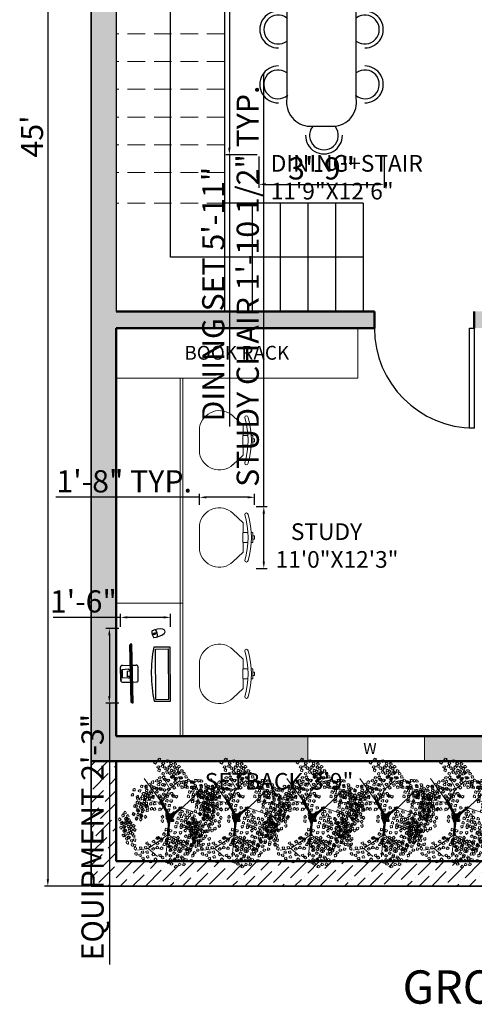
# Model space of a CAD drawing. Units: inches. Extents: x 3354 to 4308, y 1668 to 2317.
# Tile 1 of 11: x 3370 to 3534, y 1712 to 2066. Entities that reach past the tile are written whole.
import ezdxf

# ---------------------------------------------------------------- set-up
doc = ezdxf.new("R2010")
doc.units = ezdxf.units.IN
doc.linetypes.add('DASHED', pattern=[19.05, 12.7, -6.35])
for name, color, linetype, lineweight in [('A-ANNO-DIMS', 2, 'Continuous', 18), ('A-ANNO-TEXT', 7, 'Continuous', 18), ('A-AREA-IDEN', 3, 'Continuous', 18), ('A-DOOR', 3, 'Continuous', 25), ('A-EQPM', 9, 'Continuous', 18), ('A-FLOR-OVHD', 8, 'DASHED', 18), ('A-FLOR-STRS', 7, 'Continuous', 25), ('A-FURN', 8, 'Continuous', 18), ('A-GLAZ', 4, 'Continuous', 18), ('A-WALL', 7, 'Continuous', 50), ('A-WALL-PATT', 8, 'Continuous', 13), ('C-PROP', 1, 'Continuous', 35), ('L-PLNT', 84, 'Continuous', 13)]:
    doc.layers.add(name, color=color, linetype=linetype, lineweight=lineweight)
doc.layers.add('furniture', color=7, linetype='Continuous')
doc.layers.add('window', color=130, linetype='Continuous')
doc.styles.get("Standard").update_dxf_attribs({"font": 'arial.ttf'})
doc.dimstyles.new('ISO-25', dxfattribs={"dimtxt": 8, "dimasz": 2.5, "dimexe": 1.25, "dimexo": 0.625, "dimtad": 1, "dimdec": 1, "dimlunit": 3, "dimtxsty": 'Standard', "dimcen": 2.5, "dimadec": 0, "dimazin": 0, "dimtfac": 1, "dimtdec": 1, "dimtmove": 0, "dimatfit": 3, "dimfxl": 1, "dimarcsym": 0})

# ---------------------------------------------------------------- blocks, each defined once
blk = doc.blocks.new('*U3')
for p, q in [((0, 0), (0, -6)), ((36, 0), (36, -6))]:
    blk.add_line(p, q)
blk.add_lwpolyline([(0, 0), (0, 36), (1.75, 36), (1.75, 0)], close=True)
blk.add_arc((0, 0), 36, 0, 90)
blk = doc.blocks.new('UHYG')
at = {"color": 0}
for p, q in [((3464.1176, 1823.4027), (3464.1234, 1823.3981)), ((3464.1302, 1822.865), (3464.1358, 1822.8699))]:
    blk.add_line(p, q, dxfattribs=at)
at = {"layer": 'window'}
for p, q in [((3463.7616, 1823.3847), (3463.7651, 1822.8921)), ((3463.8967, 1823.3694), (3463.7767, 1823.3685)), ((3463.7767, 1823.3685), (3463.78, 1822.9085)), ((3463.8967, 1823.3694), (3463.9, 1822.9094)), ((3464.1234, 1823.3981), (3464.1358, 1822.8699)), ((3464.1078, 1823.2108), (3464.0735, 1823.21)), ((3464.1993, 1823.2129), (3464.1278, 1823.2112)), ((3464.1577, 1823.1587), (3464.1291, 1823.158)), ((3464.1576, 1823.1593), (3464.1356, 1823.1588)), ((3464.147, 1823.1745), (3464.2031, 1823.1717)), ((3464.1548, 1823.1586), (3464.1559, 1823.1106)), ((3464.1576, 1823.1593), (3464.1577, 1823.1587)), ((3464.2033, 1823.1649), (3464.2004, 1823.1649)), ((3464.2033, 1823.1643), (3464.201, 1823.1643)), ((3464.1114, 1823.0563), (3464.0771, 1823.0555)), ((3464.1588, 1823.1106), (3464.1302, 1823.11)), ((3464.2029, 1823.0584), (3464.1314, 1823.0568)), ((3464.1588, 1823.1101), (3464.1368, 1823.1096)), ((3464.1488, 1823.0943), (3464.2048, 1823.0998)), ((3464.1588, 1823.1106), (3464.1588, 1823.1101)), ((3464.2047, 1823.1066), (3464.2018, 1823.1065)), ((3464.2047, 1823.1071), (3464.2024, 1823.1071)), ((3463.9, 1822.9094), (3463.78, 1822.9085)), ((3463.8855, 1822.7631), (3463.8976, 1822.7664)), ((3463.9169, 1822.7716), (3463.8976, 1822.7664)), ((3463.9004, 1822.7713), (3463.912, 1822.7744)), ((3463.9025, 1822.7636), (3463.9141, 1822.7667)), ((3463.9169, 1822.7716), (3463.929, 1822.7748))]:
    blk.add_line(p, q, dxfattribs=at)
for points in [[(3463.9116, 1823.3858), (3463.7616, 1823.3847), (3463.7651, 1822.8921), (3463.9151, 1822.8932)], [(3464.1033, 1823.4024), (3464.1159, 1822.8647), (3464.1302, 1822.865), (3464.1176, 1823.4027), (3464.1033, 1823.4024)], [(3464.0567, 1823.1924), (3464.0595, 1823.0723)], [(3464.2004, 1823.1649), (3464.2018, 1823.1065)], [(3464.201, 1823.1643), (3464.2024, 1823.1071)], [(3464.2031, 1823.1717), (3464.2048, 1823.0998)], [(3464.2169, 1823.1961), (3464.2197, 1823.076)]]:
    blk.add_lwpolyline(points, dxfattribs=at)
for points in [[(3464.147, 1823.1745, 0.263666), (3464.137, 1823.1707), (3464.1354, 1823.1677), (3464.1356, 1823.1588)], [(3464.1488, 1823.0943, -0.263666), (3464.1387, 1823.0976), (3464.137, 1823.1006), (3464.1368, 1823.1096)]]:
    blk.add_lwpolyline(points, format="xyb", dxfattribs=at)
for centre, radius in [((3464.1159, 1823.1695), 0.00114), ((3464.2131, 1823.1967), 0.00173), ((3464.2134, 1823.1824), 0.00173), ((3464.2137, 1823.1681), 0.00173), ((3464.2141, 1823.1538), 0.00173), ((3464.1176, 1823.0979), 0.00114), ((3464.2144, 1823.1395), 0.00173), ((3464.2148, 1823.1252), 0.00173), ((3464.2151, 1823.1109), 0.00173), ((3464.2154, 1823.0966), 0.00173)]:
    blk.add_circle(centre, radius, dxfattribs=at)
for centre, radius, start, end in [((3462.7006, 1823.1307), 1.2375, 348.93511, 11.89895), ((3464.0739, 1823.1928), 0.0172, 91.34137, 181.34137), ((3464.1997, 1823.1957), 0.0172, 1.34137, 91.34137), ((3464.0767, 1823.0727), 0.0172, 181.34137, 271.34137), ((3464.2025, 1823.0756), 0.0172, 271.34137, 1.34137), ((3463.9206, 1822.6459), 0.1573, 92.25816, 129.31638), ((3464.0062, 1822.7955), 0.125, 178.78516, 211.21484), ((3463.9146, 1822.798), 0.005, 27.59246, 92.25816), ((3463.8082, 1822.7424), 0.125, 2.40754, 27.59246), ((3463.8355, 1822.7497), 0.023, 129.31638, 260.68362), ((3463.8572, 1822.8822), 0.1573, 260.68362, 297.74184), ((3463.8943, 1822.7655), 0.002, 127.29132, 262.70868), ((3463.9146, 1822.7388), 0.0355, 103.90481, 127.29132), ((3463.8985, 1822.7988), 0.0355, 262.70868, 286.09519), ((3463.9014, 1822.7674), 0.004, 105, 285), ((3463.9159, 1822.7392), 0.0355, 82.70868, 106.09519), ((3463.8998, 1822.7991), 0.0355, 283.90481, 307.29132), ((3463.913, 1822.7705), 0.004, 285, 105), ((3463.9202, 1822.7724), 0.002, 307.29132, 82.70868), ((3463.9281, 1822.7475), 0.005, 297.74184, 2.40754)]:
    blk.add_arc(centre, radius, start, end, dxfattribs=at)
blk = doc.blocks.new('A$C5D903EC3')
for p, q in [((9.01, 16.79), (5.01, 16.76)), ((9.01, 16.79), (13.02, 16.76)), ((4.51, 3.5), (1.58, 6.58)), ((13.51, 3.5), (16.44, 6.58)), ((7.51, 3.5), (4.51, 3.5)), ((10.51, 3.53), (7.51, 3.53)), ((7.51, 3.53), (7.51, 2.03)), ((10.51, 2.03), (10.51, 3.53)), ((10.51, 3.5), (13.51, 3.5)), ((7.51, 1), (7.51, 0.5)), ((7.51, 0.5), (10.51, 0.5)), ((8.51, 0.5), (8.51, 0)), ((9.51, 0), (9.51, 0.5)), ((10.51, 0.5), (10.51, 1)), ((8.51, 0), (9.51, 0))]:
    blk.add_line(p, q)
for centre, radius, start, end in [((6.1, 10.73), 6.13, 100.2152, 222.583), ((11.93, 10.73), 6.13, 317.417, 79.7848), ((2.01, 2.46), 0.5, 90, 270), ((9.01, 26.96), 25, 253.7398, 286.2602), ((9.01, 25.96), 25, 253.7398, 286.2602), ((16.01, 2.46), 0.5, 270, 90)]:
    blk.add_arc(centre, radius, start, end)
blk = doc.blocks.new('DINING')
at = {"layer": 'furniture'}
for p, q in [((67.79, 20.83), (16.8, 20.83)), ((0, 7.03), (0, -7.03)), ((84.59, -7.03), (84.59, 7.03)), ((16.8, -20.83), (67.79, -20.83))]:
    blk.add_line(p, q, dxfattribs=at)
for centre, radius, start, end in [((26.6, 26.01), 11.04, 359.28615, 180.71385), ((59.5, 26.01), 11.04, 359.28615, 180.71385), ((26.6, 26.01), 8.64, 323.1301, 216.8699), ((59.5, 26.01), 8.64, 318.78374, 216.8699), ((14.46, 6.55), 14.47, 80.69265, 178.10867), ((70.13, 6.55), 14.47, 1.89133, 99.30735), ((-5.19, 1.43), 11.04, 89.28615, 270.71385), ((90.13, 1.43), 11.04, 269.28615, 90.71385), ((-5.19, 1.43), 8.64, 53.1301, 306.8699), ((90.13, 1.43), 8.64, 233.1301, 126.8699), ((14.46, -6.55), 14.47, 181.89133, 279.30735), ((70.13, -6.55), 14.47, 260.69265, 358.10867), ((26.6, -26.01), 8.64, 143.1301, 36.8699), ((59.5, -26.01), 8.64, 143.1301, 41.21626), ((26.6, -26.01), 11.04, 179.28615, 0.71385), ((59.5, -26.01), 11.04, 179.28615, 0.71385)]:
    blk.add_arc(centre, radius, start, end, dxfattribs=at)
blk = doc.blocks.new('3DLF-C')
for points, invisible_edges in [([(-3.5, -3.5, -3.5), (3.5, -3.5, -3.5), (0, 0)], 1), ([(-3, -5, -5.6), (3, -5, -5.6), (2, -3.5, -3.5), (-2, -3.5, -3.5)], 5), ([(0, -5.7, -7.4), (1.5, -5, -5.6), (-1.5, -5, -5.6)], 2)]:
    blk.add_3dface(points, dxfattribs=dict(invisible_edges=invisible_edges))
blk = doc.blocks.new('3DLFS-C')
for p in [(-0.5, 0, 16.8), (-3, -20, -3.8), (-1.8, -11.4, 4.8), (6.5, -6.8, 12), (5.8, -22.5)]:
    blk.add_blockref('3DLF-C', p)
for p, rotation in [((-21.8, -8.2, -0.5), 330.9453959009228), ((-17.5, -13.5, 6.5), 339.0442232693679), ((-8, -6.5, 10.5), 338.5232090204596), ((12.2, -15, 3.2), 11.12918928961118), ((19.2, -4.8, 8.5), 25.76932762433872), ((21.5, -21, 1), 29.93151184050779), ((28, -11.6, 2.5), 29.93151184050779), ((-11.2, -21.8), 349.3803447238449)]:
    blk.add_blockref('3DLF-C', p, dxfattribs=dict(rotation=rotation))
blk = doc.blocks.new('3DTREE1')
at = {"extrusion": (0, -1, -2e-16)}
for p, q in [((-39.3, 39, 219.3), (-16.2, 155, 282)), ((-71.7, 67.2, 244.1), (-65.7, 127.7, 299.9)), ((-39.3, 39, 216.3), (-108, 91.9, 268.4)), ((67, 1.4, 161.3), (144.2, 5.7, 213.8))]:
    blk.add_line(p, q, dxfattribs=at)
for p, q in [((63.6, 1.4, 162.1), (106.6, 94.5, 218.9)), ((-101.1, -15.6, 180.9), (-136.1, 16, 193.3)), ((64.8, 1.4, 162.1), (123.7, -61.7, 218.9)), ((-102, -16.5, 182.6), (-131.4, -38.6, 218.5)), ((-48, -36.8, 144.2), (-101.1, -15.6, 180.9)), ((123.7, -61.7, 218.9), (147.2, -24.6, 239.4)), ((-125, -111.6, 235.9), (-53.4, -42.5, 146.8)), ((-46.7, -36.8, 144.2), (-50.1, -109.9, 182.6)), ((123.7, -61.7, 218.9), (135.2, -99.2, 233.4))]:
    blk.add_line(p, q)
at = {"extrusion": (1, 0, 0)}
blk.add_line((-21.5, -34.8, 149.8), (-37, -26.3, 257.7), dxfattribs=at)
blk.add_lwpolyline([(13.2, 14.7, -0.117832), (14.5, 13, -0.109862), (14.9, 10.8, -0.036437), (14.7, 8.3, -0.034184), (14.1, 5.7, -0.070317), (13.2, 3.9, 0.121404), (12.8, 2.7, 0.105675), (12.9, 2, 0.10563), (13.2, 1.4, 0.11787), (14.1, 0.8, 0.050289), (16.6, 0.2, 0.018663), (18.9, -0.1, 0.01497), (21.7, -0.3, 0.087147), (23.7, 0, -0.118281), (25.2, 0.2, -0.325615), (26.3, -1, -0.326103), (25.6, -2.4, -0.032273), (24.2, -3, 0.027106), (22.6, -3.7, 0.002318), (19.2, -5.3, 0.008478), (18.3, -5.8, 0.036344), (17.3, -6.4, -0.022039), (15.8, -7.5, -0.092744), (13.2, -8.5, 0.069203), (9.8, -9.6, 0.147866), (7.6, -11.8, -0.172152), (5.5, -13.5, -0.132721), (3, -13.7, 0.108842), (0, -13.9, 0.053805), (-2.2, -14.8, -0.040641), (-5.1, -16, -0.081395), (-11.5, -17.1, -0.221332), (-13.7, -16, -0.079922), (-14.4, -14.9, -0.108313), (-14.5, -13.9, -0.048517), (-14.4, -12.8, -0.02389), (-13.7, -10.5, -0.137674), (-11.4, -7.3, 0.264867), (-10.7, -5.4, 0.017693), (-10.9, -4.2, 0.00755), (-11.5, -1.5, 0.004346), (-12.4, 1.8, 0.010497), (-12.8, 3.2, 0.070056), (-13.5, 4.6, 0.023562), (-16.2, 8.3, 0.090241), (-18.7, 10.4, -0.118501), (-20.5, 12.1, -0.08154), (-20.9, 13.1, -0.126697), (-20.9, 13.8, -0.215241), (-20.5, 14.4, -0.116434), (-19.2, 14.7, -0.22855), (-18, 14.1, 0.214017), (-16.7, 13.4, 0.07524), (-15.4, 13.5, 0.190759), (-15, 13.8, 0.274563), (-14.9, 14.4, -0.2385), (-15, 15.1, -0.087445), (-14.6, 15.7, -0.110244), (-14.1, 16, -0.136741), (-13.4, 16, -0.06456), (-12, 15.5, -0.144236), (-10.5, 14.2, 0.201708), (-9.4, 13.4, 0.026586), (-7.5, 13.1, -0.015616), (-4.3, 12.5, -0.012911), (-1, 11.8, 0.016293), (1.7, 11.3, 0.100723), (3.9, 11.3, 0.063874), (7.2, 12.5, 0.158892), (8.5, 13.9, -0.171356), (9.8, 15.1, -0.140353), (11.6, 15.4, -0.14068)], format="xyb", close=True)
at = {"elevation": 87.9}
for points in [[(0.4, 3.6), (-1.1, 3.4), (-2.6, 2.5), (-3.4, 1.7), (-4.1, 0.4), (-4.3, -1.1)], [(0.4, 3.6), (1.9, 3.4), (3.4, 2.5), (4.2, 1.7), (4.9, 0.4), (5.1, -1.1)], [(0.4, -5.8), (-1.1, -5.6), (-2.6, -4.7), (-3.4, -3.9), (-4.1, -2.6), (-4.3, -1.1)], [(0.4, -5.8), (1.9, -5.6), (3.4, -4.7), (4.2, -3.9), (4.9, -2.6), (5.1, -1.1)]]:
    blk.add_lwpolyline(points, dxfattribs=at)
for centre, radius in [((0.4, -1.1), 6.83), ((0.4, -1.1, 87.9), 4.69), ((0.8, -1.1, 86.6), 3.41)]:
    blk.add_circle(centre, radius)
at = {"extrusion": (0.668965, 0, 0.743294)}
blk.add_circle((1.6, 61.5, 163.4), 2.56, dxfattribs=at)
at = {"xscale": 1.706666666666666, "yscale": 1.706666666666666, "zscale": 1.706666666666666}
for name, p, rotation in [('3DLFS-C', (-50.3, 113, 288.1), 217.0355451173859), ('3DLFS-C', (-13.6, 138.7, 209.1), 180), ('3DLFS-C', (-89, 85.2, 227), 217.0355451173859), ('3DLFS-C', (-90.3, 99.3, 187.4), 241.10908773184), ('3DLFS-C', (-30.5, 83, 187.3), 217.0355451173859), ('3DLFS-C', (1, 105.9, 248.4), 180), ('3DLFS-C', (21.9, 87, 153.2), 127.0355451173859), ('3DLFS-C', (41.5, 81.2, 271.8), 127.0355451173859), ('3DLFS-C', (68.8, 96.4, 191.6), 127.0355451173859), ('3DLFS-C', (-80.4, 50.7, 249.2), 217.0355451173859), ('3DLFS-C', (28.8, 51.1, 172), 217.0355451173859), ('3DLFS-C', (126.8, 45.3, 236), 116.7371100578058), ('3DLFS-C', (-108.7, 24.8, 134.8), 241.10908773184), ('3DLFS-C', (19.6, 23.1, 316.2), 217.0355451173859), ('3DLFS-C', (64.3, 39.8, 138.3), 90), ('3DLFS-C', (73.7, 39.8, 300.3), 90), ('3DLFS-C', (113.3, 18.1, 166.2), 105.1767250495332), ('3DLFS-C', (-141, -10.4, 198.6), 274.426310174705), ('3DLFS-C', (-101.5, -0.4, 274.2), 274.426310174705), ('3DLFS-C', (41.6, -10, 304.8), 127.0355451173859), ('3DLFS-C', (-154.1, -35.2, 230.9), 260.280514680602), ('3DLFS-C', (-54.5, -35.2, 179.4), 274.426310174705), ('3DLFS-C', (-36, -5.1, 325.5), 311.4618552920909), ('3DLFS-C', (76.2, -35.1, 240.2), 105.1767250495332), ('3DLFS-C', (-90, -43.3, 295.7), 311.4618552920909), ('3DLF-C', (-20.6, -4.1, 353.7), 319.1446237411043), ('3DLF-C', (14.1, -21.6, 363.3), 46.3875157474432), ('3DLFS-C', (116.7, -67.8, 211.5), 68.14117993214732), ('3DLFS-C', (-59.6, -89, 158.7), 294.8881552746311), ('3DLFS-C', (-17.8, -65, 244.3), 342.4928092333246), ('3DLFS-C', (-17.8, -80.2, 257.5), 342.4928092333246), ('3DLFS-C', (-25.2, -86.2, 179.4), 351.3217393776923), ('3DLFS-C', (48.4, -119.8, 204.2), 20.68147253157148), ('3DLFS-C', (62.7, -113.9, 272.2), 19.52835435071045), ('3DLFS-C', (38.6, -131.8, 232.1), 19.52835435071045)]:
    blk.add_blockref(name, p, dxfattribs=dict(at, rotation=rotation))
blk.add_blockref('3DLF-C', (3.3, -21.6, 352.8), dxfattribs=at)
mesh = blk.add_polymesh((2, 36), dxfattribs=dict(n_close=True))
for k, corner in enumerate([(-1.5, 0.6, 84.1), (-1, 1, 84.1), (-0.5, 1.4, 84.1), (0.1, 1.6, 84.1), (0.6, 1.7, 84.1), (1.2, 1.7, 84.1), (1.8, 1.6, 84.1), (2.4, 1.4, 84.1), (2.9, 1.1, 84.1), (3.4, 0.8, 84.1), (3.8, 0.3, 84.1), (4.1, -0.2, 84.1), (4.3, -0.7, 84.1), (4.4, -1.3, 84.1), (4.4, -1.9, 84.1), (4.3, -2.5, 84.1), (4.2, -3.1, 84.1), (3.9, -3.6, 84.1), (3.5, -4.1, 84.1), (3.1, -4.4, 84.1), (2.5, -4.8, 84.1), (2, -5, 84.1), (1.4, -5.1, 84.1), (0.8, -5.1, 84.1), (0.2, -5, 84.1), (-0.3, -4.8, 84.1), (-0.9, -4.5, 84.1), (-1.3, -4.2, 84.1), (-1.7, -3.7, 84.1), (-2, -3.2, 84.1), (-2.2, -2.7, 84.1), (-2.4, -2.1, 84.1), (-2.4, -1.5, 84.1), (-2.3, -0.9, 84.1), (-2.1, -0.3, 84.1), (-1.8, 0.2, 84.1), (-38.4, 38.9, 216.7), (-38.2, 38.6, 217), (-38, 38.3, 217.3), (-37.9, 38, 217.6), (-37.9, 37.6, 217.8), (-38, 37.2, 218.1), (-38.1, 36.8, 218.2), (-38.3, 36.4, 218.4), (-38.5, 36, 218.4), (-38.8, 35.7, 218.5), (-39.1, 35.4, 218.4), (-39.5, 35.1, 218.4), (-39.8, 34.9, 218.2), (-40.2, 34.8, 218.1), (-40.6, 34.7, 217.8), (-41, 34.7, 217.6), (-41.3, 34.8, 217.3), (-41.7, 34.9, 217), (-41.9, 35.1, 216.7), (-42.1, 35.4, 216.4), (-42.3, 35.7, 216.2), (-42.4, 36.1, 215.9), (-42.4, 36.4, 215.6), (-42.4, 36.8, 215.4), (-42.2, 37.2, 215.3), (-42.1, 37.6, 215.1), (-41.8, 38, 215.1), (-41.5, 38.3, 215), (-41.2, 38.6, 215.1), (-40.9, 38.9, 215.1), (-40.5, 39.1, 215.3), (-40.1, 39.2, 215.4), (-39.7, 39.3, 215.6), (-39.3, 39.3, 215.9), (-39, 39.2, 216.2), (-38.7, 39.1, 216.4)]):
    mesh.set_mesh_vertex(divmod(k, 36), corner)
mesh = blk.add_polymesh((2, 36), dxfattribs=dict(n_close=True))
for k, corner in enumerate([(-1.5, 0.6, 84.1), (-1, 1, 84.1), (-0.5, 1.4, 84.1), (0.1, 1.6, 84.1), (0.6, 1.7, 84.1), (1.2, 1.7, 84.1), (1.8, 1.6, 84.1), (2.4, 1.4, 84.1), (2.9, 1.1, 84.1), (3.4, 0.8, 84.1), (3.8, 0.3, 84.1), (4.1, -0.2, 84.1), (4.3, -0.7, 84.1), (4.4, -1.3, 84.1), (4.4, -1.9, 84.1), (4.3, -2.5, 84.1), (4.2, -3.1, 84.1), (3.9, -3.6, 84.1), (3.5, -4.1, 84.1), (3.1, -4.4, 84.1), (2.5, -4.8, 84.1), (2, -5, 84.1), (1.4, -5.1, 84.1), (0.8, -5.1, 84.1), (0.2, -5, 84.1), (-0.3, -4.8, 84.1), (-0.9, -4.5, 84.1), (-1.3, -4.2, 84.1), (-1.7, -3.7, 84.1), (-2, -3.2, 84.1), (-2.2, -2.7, 84.1), (-2.4, -2.1, 84.1), (-2.4, -1.5, 84.1), (-2.3, -0.9, 84.1), (-2.1, -0.3, 84.1), (-1.8, 0.2, 84.1), (-38.4, 38.9, 216.7), (-38.2, 38.6, 217), (-38, 38.3, 217.3), (-37.9, 38, 217.6), (-37.9, 37.6, 217.8), (-38, 37.2, 218.1), (-38.1, 36.8, 218.2), (-38.3, 36.4, 218.4), (-38.5, 36, 218.4), (-38.8, 35.7, 218.5), (-39.1, 35.4, 218.4), (-39.5, 35.1, 218.4), (-39.8, 34.9, 218.2), (-40.2, 34.8, 218.1), (-40.6, 34.7, 217.8), (-41, 34.7, 217.6), (-41.3, 34.8, 217.3), (-41.7, 34.9, 217), (-41.9, 35.1, 216.7), (-42.1, 35.4, 216.4), (-42.3, 35.7, 216.2), (-42.4, 36.1, 215.9), (-42.4, 36.4, 215.6), (-42.4, 36.8, 215.4), (-42.2, 37.2, 215.3), (-42.1, 37.6, 215.1), (-41.8, 38, 215.1), (-41.5, 38.3, 215), (-41.2, 38.6, 215.1), (-40.9, 38.9, 215.1), (-40.5, 39.1, 215.3), (-40.1, 39.2, 215.4), (-39.7, 39.3, 215.6), (-39.3, 39.3, 215.9), (-39, 39.2, 216.2), (-38.7, 39.1, 216.4)]):
    mesh.set_mesh_vertex(divmod(k, 36), corner)
mesh = blk.add_polymesh((2, 36), dxfattribs=dict(n_close=True))
for k, corner in enumerate([(-1.5, -2.8, 84.1), (-1.9, -2.3, 84.1), (-2.1, -1.8, 84.1), (-2.3, -1.2, 84.1), (-2.4, -0.7, 84.1), (-2.3, -0.1, 84.1), (-2.2, 0.5, 84.1), (-2, 1.1, 84.1), (-1.6, 1.6, 84.1), (-1.2, 2, 84.1), (-0.8, 2.4, 84.1), (-0.2, 2.6, 84.1), (0.3, 2.8, 84.1), (0.9, 2.9, 84.1), (1.5, 2.8, 84.1), (2.1, 2.7, 84.1), (2.6, 2.5, 84.1), (3.1, 2.1, 84.1), (3.6, 1.7, 84.1), (3.9, 1.3, 84.1), (4.2, 0.7, 84.1), (4.4, 0.2, 84.1), (4.5, -0.4, 84.1), (4.4, -1, 84.1), (4.3, -1.6, 84.1), (4.1, -2.1, 84.1), (3.7, -2.6, 84.1), (3.3, -3.1, 84.1), (2.8, -3.4, 84.1), (2.3, -3.7, 84.1), (1.7, -3.9, 84.1), (1.2, -4, 84.1), (0.6, -3.9, 84.1), (0, -3.8, 84.1), (-0.6, -3.6, 84.1), (-1.1, -3.2, 84.1), (-55.7, -36.2, 146.8), (-55.4, -36, 147.1), (-55.1, -35.9, 147.4), (-54.7, -35.8, 147.6), (-54.3, -35.8, 147.9), (-54, -35.9, 148.1), (-53.6, -36.1, 148.3), (-53.2, -36.3, 148.4), (-52.8, -36.5, 148.5), (-52.5, -36.9, 148.5), (-52.3, -37.2, 148.5), (-52, -37.6, 148.4), (-51.9, -38, 148.3), (-51.8, -38.4, 148.1), (-51.7, -38.8, 147.9), (-51.8, -39.1, 147.6), (-51.9, -39.5, 147.4), (-52, -39.8, 147.1), (-52.2, -40, 146.8), (-52.5, -40.2, 146.5), (-52.8, -40.3, 146.2), (-53.2, -40.4, 145.9), (-53.5, -40.4, 145.7), (-53.9, -40.3, 145.5), (-54.3, -40.2, 145.3), (-54.7, -40, 145.2), (-55, -39.7, 145.1), (-55.4, -39.4, 145.1), (-55.6, -39, 145.1), (-55.9, -38.7, 145.2), (-56, -38.3, 145.3), (-56.1, -37.9, 145.5), (-56.2, -37.5, 145.7), (-56.1, -37.1, 145.9), (-56, -36.8, 146.2), (-55.9, -36.5, 146.5)]):
    mesh.set_mesh_vertex(divmod(k, 36), corner)
mesh = blk.add_polymesh((2, 36), dxfattribs=dict(n_close=True))
for k, corner in enumerate([(-1.5, -2.8, 84.1), (-1.9, -2.3, 84.1), (-2.1, -1.8, 84.1), (-2.3, -1.2, 84.1), (-2.4, -0.7, 84.1), (-2.3, -0.1, 84.1), (-2.2, 0.5, 84.1), (-2, 1.1, 84.1), (-1.6, 1.6, 84.1), (-1.2, 2, 84.1), (-0.8, 2.4, 84.1), (-0.2, 2.6, 84.1), (0.3, 2.8, 84.1), (0.9, 2.9, 84.1), (1.5, 2.8, 84.1), (2.1, 2.7, 84.1), (2.6, 2.5, 84.1), (3.1, 2.1, 84.1), (3.6, 1.7, 84.1), (3.9, 1.3, 84.1), (4.2, 0.7, 84.1), (4.4, 0.2, 84.1), (4.5, -0.4, 84.1), (4.4, -1, 84.1), (4.3, -1.6, 84.1), (4.1, -2.1, 84.1), (3.7, -2.6, 84.1), (3.3, -3.1, 84.1), (2.8, -3.4, 84.1), (2.3, -3.7, 84.1), (1.7, -3.9, 84.1), (1.2, -4, 84.1), (0.6, -3.9, 84.1), (0, -3.8, 84.1), (-0.6, -3.6, 84.1), (-1.1, -3.2, 84.1), (-53.9, -39.6, 146.8), (-53.7, -39.4, 147.1), (-53.4, -39.3, 147.4), (-53, -39.3, 147.6), (-52.6, -39.3, 147.9), (-52.3, -39.3, 148.1), (-51.9, -39.5, 148.3), (-51.5, -39.7, 148.4), (-51.1, -40, 148.5), (-50.8, -40.3, 148.5), (-50.5, -40.6, 148.5), (-50.3, -41, 148.4), (-50.2, -41.4, 148.3), (-50.1, -41.8, 148.1), (-50, -42.2, 147.9), (-50, -42.6, 147.6), (-50.1, -42.9, 147.4), (-50.3, -43.2, 147.1), (-50.5, -43.4, 146.8), (-50.8, -43.6, 146.5), (-51.1, -43.8, 146.2), (-51.5, -43.8, 145.9), (-51.8, -43.8, 145.7), (-52.2, -43.7, 145.5), (-52.6, -43.6, 145.3), (-53, -43.4, 145.2), (-53.3, -43.1, 145.1), (-53.7, -42.8, 145.1), (-53.9, -42.5, 145.1), (-54.2, -42.1, 145.2), (-54.3, -41.7, 145.3), (-54.4, -41.3, 145.5), (-54.5, -40.9, 145.7), (-54.4, -40.5, 145.9), (-54.3, -40.2, 146.2), (-54.2, -39.9, 146.5)]):
    mesh.set_mesh_vertex(divmod(k, 36), corner)
mesh = blk.add_polymesh((2, 36), dxfattribs=dict(n_close=True))
for k, corner in enumerate([(7.2, -1.1), (7.1, 0.1), (6.8, 1.2), (6.3, 2.3), (5.6, 3.3), (4.8, 4.1), (3.8, 4.8), (2.7, 5.3), (1.6, 5.6), (0.4, 5.7), (-0.8, 5.6), (-1.9, 5.3), (-3, 4.8), (-4, 4.1), (-4.8, 3.3), (-5.5, 2.3), (-6, 1.2), (-6.3, 0.1), (-6.4, -1.1), (-6.3, -2.3), (-6, -3.4), (-5.5, -4.5), (-4.8, -5.5), (-4, -6.3), (-3, -7), (-1.9, -7.5), (-0.8, -7.8), (0.4, -7.9), (1.6, -7.8), (2.7, -7.5), (3.8, -7), (4.8, -6.3), (5.6, -5.5), (6.3, -4.5), (6.8, -3.4), (7.1, -2.3), (9.4, 14.9, -23.9), (6.4, 12.2, -23.9), (2.5, 11.2, -23.9), (-1.5, 11.9, -23.9), (-5.5, 12.8, -23.9), (-9.6, 13.4, -23.9), (-12.8, 15.8, -23.9), (-15, 13.7, -23.9), (-18.7, 14.6, -23.9), (-20.6, 12.4, -23.9), (-17.6, 9.7, -23.9), (-14.9, 6.6, -23.9), (-12.8, 3.1, -23.9), (-11.7, -0.8, -23.9), (-10.8, -4.8, -23.9), (-12.4, -8.3, -23.9), (-14.1, -11.9, -23.9), (-13.9, -15.8, -23.9), (-10.2, -17, -23.9), (-6.2, -16.4, -23.9), (-2.4, -14.9, -23.9), (1.5, -13.7, -23.9), (5.6, -13.5, -23.9), (8.4, -10.6, -23.9), (12, -8.8, -23.9), (15.9, -7.5, -23.9), (19.3, -5.3, -23.9), (23, -3.5, -23.9), (26.3, -1.4, -23.9), (23.2, -0.1, -23.9), (19.2, -0.1, -23.9), (15.1, 0.5, -23.9), (12.9, 3.3, -23.9), (14.4, 7, -23.9), (14.9, 11.1, -23.9), (13.2, 14.7, -23.9)]):
    mesh.set_mesh_vertex(divmod(k, 36), corner)
mesh = blk.add_polymesh((2, 36), dxfattribs=dict(n_close=True))
for k, corner in enumerate([(7.2, -1.1), (7.1, 0.1), (6.8, 1.2), (6.3, 2.3), (5.6, 3.3), (4.8, 4.1), (3.8, 4.8), (2.7, 5.3), (1.6, 5.6), (0.4, 5.7), (-0.8, 5.6), (-1.9, 5.3), (-3, 4.8), (-4, 4.1), (-4.8, 3.3), (-5.5, 2.3), (-6, 1.2), (-6.3, 0.1), (-6.4, -1.1), (-6.3, -2.3), (-6, -3.4), (-5.5, -4.5), (-4.8, -5.5), (-4, -6.3), (-3, -7), (-1.9, -7.5), (-0.8, -7.8), (0.4, -7.9), (1.6, -7.8), (2.7, -7.5), (3.8, -7), (4.8, -6.3), (5.6, -5.5), (6.3, -4.5), (6.8, -3.4), (7.1, -2.3), (5.1, -1.1, 87.9), (5, -0.3, 87.9), (4.8, 0.5, 87.9), (4.5, 1.2, 87.9), (4, 1.9, 87.9), (3.4, 2.5, 87.9), (2.8, 3, 87.9), (2, 3.3, 87.9), (1.2, 3.5, 87.9), (0.4, 3.6, 87.9), (-0.4, 3.5, 87.9), (-1.2, 3.3, 87.9), (-1.9, 3, 87.9), (-2.6, 2.5, 87.9), (-3.2, 1.9, 87.9), (-3.7, 1.2, 87.9), (-4, 0.5, 87.9), (-4.2, -0.3, 87.9), (-4.3, -1.1, 87.9), (-4.2, -1.9, 87.9), (-4, -2.7, 87.9), (-3.7, -3.5, 87.9), (-3.2, -4.1, 87.9), (-2.6, -4.7, 87.9), (-1.9, -5.2, 87.9), (-1.2, -5.5, 87.9), (-0.4, -5.7, 87.9), (0.4, -5.8, 87.9), (1.2, -5.7, 87.9), (2, -5.5, 87.9), (2.8, -5.2, 87.9), (3.4, -4.7, 87.9), (4, -4.1, 87.9), (4.5, -3.5, 87.9), (4.8, -2.7, 87.9), (5, -1.9, 87.9)]):
    mesh.set_mesh_vertex(divmod(k, 36), corner)
mesh = blk.add_polymesh((2, 36), dxfattribs=dict(n_close=True))
for k, corner in enumerate([(4.2, -1.1, 86.6), (4.2, -0.5, 86.6), (4, 0.1, 86.6), (3.8, 0.6, 86.6), (3.4, 1.1, 86.6), (3, 1.5, 86.6), (2.5, 1.8, 86.6), (2, 2.1, 86.6), (1.4, 2.2, 86.6), (0.8, 2.3, 86.6), (0.2, 2.2, 86.6), (-0.3, 2.1, 86.6), (-0.9, 1.8, 86.6), (-1.4, 1.5, 86.6), (-1.8, 1.1, 86.6), (-2.1, 0.6, 86.6), (-2.4, 0.1, 86.6), (-2.5, -0.5, 86.6), (-2.6, -1.1, 86.6), (-2.5, -1.7, 86.6), (-2.4, -2.3, 86.6), (-2.1, -2.8, 86.6), (-1.8, -3.3, 86.6), (-1.4, -3.7, 86.6), (-0.9, -4.1, 86.6), (-0.3, -4.3, 86.6), (0.2, -4.5, 86.6), (0.8, -4.5, 86.6), (1.4, -4.5, 86.6), (2, -4.3, 86.6), (2.5, -4.1, 86.6), (3, -3.7, 86.6), (3.4, -3.3, 86.6), (3.8, -2.8, 86.6), (4, -2.3, 86.6), (4.2, -1.7, 86.6), (63.6, 4.2, 162.6), (63.3, 4.1, 162.9), (62.9, 4, 163.1), (62.6, 3.8, 163.4), (62.4, 3.6, 163.7), (62.1, 3.2, 163.9), (61.9, 2.9, 164), (61.8, 2.5, 164.2), (61.7, 2, 164.2), (61.7, 1.6, 164.3), (61.7, 1.2, 164.2), (61.8, 0.7, 164.2), (61.9, 0.3, 164), (62.1, 0, 163.9), (62.4, -0.4, 163.7), (62.6, -0.6, 163.4), (62.9, -0.8, 163.1), (63.3, -0.9, 162.9), (63.6, -1, 162.6), (63.9, -0.9, 162.3), (64.2, -0.8, 162), (64.5, -0.6, 161.7), (64.8, -0.4, 161.5), (65.1, 0, 161.2), (65.2, 0.3, 161.1), (65.4, 0.7, 160.9), (65.5, 1.2, 160.9), (65.5, 1.6, 160.8), (65.5, 2, 160.9), (65.4, 2.5, 160.9), (65.2, 2.9, 161.1), (65.1, 3.2, 161.2), (64.8, 3.6, 161.5), (64.5, 3.8, 161.7), (64.2, 4, 162), (63.9, 4.1, 162.3)]):
    mesh.set_mesh_vertex(divmod(k, 36), corner)
blk = doc.blocks.new('*D50')
at = {"layer": 'A-ANNO-DIMS', "color": 0, "lineweight": -2, "transparency": 16777216}
for p, q in [((3395.65, 2294.3), (3379.37, 2294.3)), ((3380.62, 2291.8), (3380.62, 1756.8)), ((3395.65, 1754.3), (3379.37, 1754.3))]:
    blk.add_line(p, q, dxfattribs=at)
at = {"layer": 'A-ANNO-DIMS', "color": 0, "transparency": 16777216}
for points in [[(3380.2, 2291.8), (3381.04, 2291.8), (3380.62, 2294.3)], [(3380.2, 1756.8), (3381.04, 1756.8), (3380.62, 1754.3)]]:
    blk.add_solid(points, dxfattribs=at)
at = {"layer": 'Defpoints', "color": 0, "transparency": 16777216}
for p in [(3396.28, 2294.3), (3380.62, 1754.3), (3396.28, 1754.3)]:
    blk.add_point(p, dxfattribs=at)
at = {"layer": 'A-ANNO-DIMS', "color": 0, "transparency": 16777216, "insert": (3375.93, 2024.3), "char_height": 8, "attachment_point": 5, "rotation": 90}
blk.add_mtext("45'", dxfattribs=at)
blk = doc.blocks.new('*D58')
at = {"layer": 'A-ANNO-DIMS', "color": 0, "lineweight": -2, "transparency": 16777216}
for p, q in [((3458.43, 1891.03), (3458.43, 2047.22)), ((3455.72, 1891.03), (3459.68, 1891.03)), ((3458.43, 1871.24), (3458.43, 1888.53)), ((3455.72, 1868.74), (3459.68, 1868.74))]:
    blk.add_line(p, q, dxfattribs=at)
at = {"layer": 'A-ANNO-DIMS', "color": 0, "transparency": 16777216}
for points in [[(3458.02, 1888.53), (3458.85, 1888.53), (3458.43, 1891.03)], [(3458.02, 1871.24), (3458.85, 1871.24), (3458.43, 1868.74)]]:
    blk.add_solid(points, dxfattribs=at)
at = {"layer": 'Defpoints', "color": 0, "transparency": 16777216}
for p in [(3455.09, 1891.03), (3458.43, 1891.03), (3455.09, 1868.74)]:
    blk.add_point(p, dxfattribs=at)
at = {"layer": 'A-ANNO-DIMS', "color": 0, "transparency": 16777216, "insert": (3453.67, 1970.38), "char_height": 8, "attachment_point": 5, "rotation": 90}
blk.add_mtext('STUDY CHAIR 1\'-10 1/2" TYP.', dxfattribs=at)
blk = doc.blocks.new('*D59')
at = {"layer": 'A-ANNO-DIMS', "color": 0, "lineweight": -2, "transparency": 16777216}
for p, q in [((3435.26, 1894.38), (3383.5, 1894.38)), ((3435.26, 1891.66), (3435.26, 1895.63)), ((3452.59, 1894.38), (3437.76, 1894.38)), ((3455.09, 1891.66), (3455.09, 1895.63))]:
    blk.add_line(p, q, dxfattribs=at)
at = {"layer": 'A-ANNO-DIMS', "color": 0, "transparency": 16777216}
for points in [[(3437.76, 1894.79), (3437.76, 1893.96), (3435.26, 1894.38)], [(3452.59, 1894.79), (3452.59, 1893.96), (3455.09, 1894.38)]]:
    blk.add_solid(points, dxfattribs=at)
at = {"layer": 'Defpoints', "color": 0, "transparency": 16777216}
for p in [(3435.26, 1894.38), (3435.26, 1891.03), (3455.09, 1891.03)]:
    blk.add_point(p, dxfattribs=at)
at = {"layer": 'A-ANNO-DIMS', "color": 0, "transparency": 16777216, "insert": (3408.13, 1899.09), "char_height": 8, "attachment_point": 5}
blk.add_mtext('1\'-8" TYP.', dxfattribs=at)
blk = doc.blocks.new('*D76')
at = {"layer": 'A-ANNO-DIMS', "color": 0, "lineweight": -2, "transparency": 16777216}
for p, q in [((3406.18, 1847.12), (3401.53, 1847.12)), ((3402.78, 1844.62), (3402.78, 1822.8)), ((3406.18, 1820.3), (3401.53, 1820.3)), ((3402.78, 1820.3), (3402.78, 1726.16))]:
    blk.add_line(p, q, dxfattribs=at)
at = {"layer": 'A-ANNO-DIMS', "color": 0, "transparency": 16777216}
for points in [[(3402.36, 1844.62), (3403.2, 1844.62), (3402.78, 1847.12)], [(3402.36, 1822.8), (3403.2, 1822.8), (3402.78, 1820.3)]]:
    blk.add_solid(points, dxfattribs=at)
at = {"layer": 'Defpoints', "color": 0, "transparency": 16777216}
for p in [(3406.8, 1847.12), (3402.78, 1820.3), (3406.8, 1820.3)]:
    blk.add_point(p, dxfattribs=at)
at = {"layer": 'A-ANNO-DIMS', "color": 0, "transparency": 16777216, "insert": (3397.77, 1771.98), "char_height": 8, "attachment_point": 5, "rotation": 90}
blk.add_mtext('EQUIPMENT 2\'-3"', dxfattribs=at)
blk = doc.blocks.new('*D77')
at = {"layer": 'A-ANNO-DIMS', "color": 0, "lineweight": -2, "transparency": 16777216}
for p, q in [((3406.8, 1851.14), (3382.54, 1851.14)), ((3406.8, 1847.74), (3406.8, 1852.39)), ((3422.34, 1851.14), (3409.3, 1851.14)), ((3424.84, 1847.74), (3424.84, 1852.39))]:
    blk.add_line(p, q, dxfattribs=at)
at = {"layer": 'A-ANNO-DIMS', "color": 0, "transparency": 16777216}
for points in [[(3409.3, 1851.56), (3409.3, 1850.73), (3406.8, 1851.14)], [(3422.34, 1851.56), (3422.34, 1850.73), (3424.84, 1851.14)]]:
    blk.add_solid(points, dxfattribs=at)
at = {"layer": 'Defpoints', "color": 0, "transparency": 16777216}
for p in [(3406.8, 1851.14), (3406.8, 1847.12), (3424.84, 1847.12)]:
    blk.add_point(p, dxfattribs=at)
at = {"layer": 'A-ANNO-DIMS', "color": 0, "transparency": 16777216, "insert": (3393.42, 1855.85), "char_height": 8, "attachment_point": 5}
blk.add_mtext('1\'-6"', dxfattribs=at)
blk = doc.blocks.new('*D88')
at = {"layer": 'A-ANNO-DIMS', "color": 0, "lineweight": -2, "transparency": 16777216}
for p, q in [((3405.28, 2080.67), (3405.28, 2074.65)), ((3441.28, 2080.67), (3441.28, 2074.65)), ((3407.78, 2075.9), (3438.78, 2075.9)), ((3441.28, 2075.9), (3543.5, 2075.9))]:
    blk.add_line(p, q, dxfattribs=at)
at = {"layer": 'A-ANNO-DIMS', "color": 0, "transparency": 16777216}
for points in [[(3407.78, 2076.31), (3407.78, 2075.48), (3405.28, 2075.9)], [(3438.78, 2076.31), (3438.78, 2075.48), (3441.28, 2075.9)]]:
    blk.add_solid(points, dxfattribs=at)
at = {"layer": 'Defpoints', "color": 0, "transparency": 16777216}
for p in [(3405.28, 2081.3), (3441.28, 2081.3), (3441.28, 2075.9)]:
    blk.add_point(p, dxfattribs=at)
at = {"layer": 'A-ANNO-DIMS', "color": 0, "transparency": 16777216, "insert": (3493.64, 2080.66), "char_height": 8, "attachment_point": 5}
blk.add_mtext('RANGE OVEN 3\'-0"', dxfattribs=at)
blk = doc.blocks.new('*D90')
at = {"layer": 'A-ANNO-DIMS', "color": 0, "lineweight": -2, "transparency": 16777216}
for p, q in [((3456.06, 2088.83), (3444.77, 2088.83)), ((3446.02, 2086.33), (3446.02, 2020.22)), ((3456.06, 2017.72), (3444.77, 2017.72)), ((3446.02, 2017.72), (3446.02, 1919.83))]:
    blk.add_line(p, q, dxfattribs=at)
at = {"layer": 'A-ANNO-DIMS', "color": 0, "transparency": 16777216}
for points in [[(3445.6, 2086.33), (3446.44, 2086.33), (3446.02, 2088.83)], [(3445.6, 2020.22), (3446.44, 2020.22), (3446.02, 2017.72)]]:
    blk.add_solid(points, dxfattribs=at)
at = {"layer": 'Defpoints', "color": 0, "transparency": 16777216}
for p in [(3456.69, 2088.83), (3446.02, 2017.72), (3456.69, 2017.72)]:
    blk.add_point(p, dxfattribs=at)
at = {"layer": 'A-ANNO-DIMS', "color": 0, "transparency": 16777216, "insert": (3441.26, 1967.53), "char_height": 8, "attachment_point": 5, "rotation": 90}
blk.add_mtext('DINING SET 5\'-11"', dxfattribs=at)
blk = doc.blocks.new('*D91')
at = {"layer": 'A-ANNO-DIMS', "color": 0, "lineweight": -2, "transparency": 16777216}
for p, q in [((3456.69, 2017.1), (3456.69, 2005.81)), ((3501.79, 2017.1), (3501.79, 2005.81)), ((3459.19, 2007.06), (3499.29, 2007.06))]:
    blk.add_line(p, q, dxfattribs=at)
at = {"layer": 'A-ANNO-DIMS', "color": 0, "transparency": 16777216}
for points in [[(3459.19, 2007.48), (3459.19, 2006.64), (3456.69, 2007.06)], [(3499.29, 2007.48), (3499.29, 2006.64), (3501.79, 2007.06)]]:
    blk.add_solid(points, dxfattribs=at)
at = {"layer": 'Defpoints', "color": 0, "transparency": 16777216}
for p in [(3456.69, 2017.72), (3501.79, 2017.72), (3501.79, 2007.06)]:
    blk.add_point(p, dxfattribs=at)
at = {"layer": 'A-ANNO-DIMS', "color": 0, "transparency": 16777216, "insert": (3479.24, 2011.77), "char_height": 8, "attachment_point": 5}
blk.add_mtext('3\'-9"', dxfattribs=at)

msp = doc.modelspace()

# ---------------------------------------------------------------- hatches: boundary and pattern name
at = {"layer": 'A-WALL-PATT', "transparency": 33554687}
h = msp.add_hatch(color=256, dxfattribs=at)
h.dxf.hatch_style = 1
h.paths.add_polyline_path([(3546.28, 1829.3), (3552.28, 1829.3), (3552.28, 1838.3), (3546.28, 1838.3), (3546.28, 1910.3), (3582.28, 1910.3), (3582.28, 1919.3), (3546.28, 1919.3), (3546.28, 1961.3), (3534.28, 1961.3), (3534.28, 1955.3), (3537.28, 1955.3), (3537.28, 1808.3), (3516.28, 1808.3), (3516.28, 1799.3), (3546.28, 1799.3)])
h.paths.add_polyline_path([(3672.28, 1919.3), (3656.51, 1919.3), (3630.28, 1919.3), (3630.28, 1910.3), (3642.28, 1910.3), (3642.28, 1838.3), (3630.28, 1838.3), (3630.28, 1835.3), (3630.28, 1829.3), (3642.28, 1829.3), (3642.28, 1799.3), (3651.28, 1799.3), (3651.28, 1910.3), (3672.28, 1910.3)])
h.paths.add_polyline_path([(3744.28, 1959.8), (3735.28, 1959.8), (3735.28, 1923.23), (3735.28, 1919.3), (3714.28, 1919.3), (3714.28, 1910.3), (3744.28, 1910.3)])
h.paths.add_polyline_path([(3744.28, 2072.3), (3735.28, 2072.3), (3735.28, 2031.8), (3744.28, 2031.8)])
h.paths.add_polyline_path([(3744.28, 2150.3), (3735.28, 2150.3), (3735.28, 2108.3), (3744.28, 2108.3)])
h.paths.add_polyline_path([(3744.28, 2258.3), (3705.28, 2258.3), (3705.28, 2249.3), (3735.28, 2249.3), (3735.28, 2210.3), (3744.28, 2210.3)])
h.paths.add_polyline_path([(3633.28, 2258.3), (3583.78, 2258.3), (3583.78, 2249.3), (3588.24, 2249.3), (3597.28, 2249.3), (3597.28, 2165.3), (3594.28, 2165.3), (3594.28, 2159.3), (3597.28, 2159.3), (3597.28, 2117.3), (3594.28, 2117.3), (3594.28, 2111.3), (3603.28, 2111.3), (3603.28, 2249.3), (3633.28, 2249.3)])
h.paths.add_polyline_path([(3559.78, 2258.3), (3492.28, 2258.3), (3492.28, 2249.3), (3537.28, 2249.3), (3537.28, 2117.3), (3534.28, 2117.3), (3534.28, 2111.3), (3564.28, 2111.3), (3564.28, 2117.3), (3546.28, 2117.3), (3546.28, 2159.3), (3564.28, 2159.3), (3564.28, 2165.3), (3546.28, 2165.3), (3546.28, 2249.3), (3559.78, 2249.3)])
h.paths.add_polyline_path([(3450.28, 2258.3), (3396.28, 2258.3), (3396.28, 1799.3), (3474.28, 1799.3), (3474.28, 1808.3), (3405.28, 1808.3), (3405.28, 1955.3), (3498.28, 1955.3), (3498.28, 1961.3), (3405.28, 1961.3), (3405.28, 2111.3), (3498.28, 2111.3), (3498.28, 2117.3), (3405.28, 2117.3), (3405.28, 2249.3), (3450.28, 2249.3)])
h.paths.add_polyline_path([(3582.28, 1838.3), (3576.28, 1838.3), (3576.28, 1829.3), (3582.28, 1829.3)], flags=17)
h = msp.add_hatch(dxfattribs=at)
h.set_pattern_fill('ANSI36', color=256)
h.paths.add_polyline_path([(3576.28, 1763.3), (3405.28, 1763.3), (3405.28, 1799.3), (3396.28, 1799.3), (3396.28, 1754.3), (3576.28, 1754.3)])

# ---------------------------------------------------------------- linework, layer by layer
at = {"layer": 'A-FLOR-OVHD', "ltscale": 0.5}
for p, q in [((3444.28, 2061.3), (3405.28, 2061.3)), ((3444.28, 2051.3), (3405.28, 2051.3)), ((3444.28, 2041.3), (3405.28, 2041.3)), ((3444.28, 2031.3), (3405.28, 2031.3)), ((3444.28, 2021.3), (3405.28, 2021.3)), ((3444.28, 2011.3), (3405.28, 2011.3)), ((3444.28, 2000.3), (3405.28, 2000.3))]:
    msp.add_line(p, q, dxfattribs=at)
at = {"layer": 'A-FLOR-STRS'}
for p, q in [((3405.28, 2111.3), (3405.28, 1961.3)), ((3444.28, 2072.3), (3444.28, 1961.3)), ((3494.28, 2000.3), (3444.28, 2000.3)), ((3454.28, 2000.3), (3454.28, 1961.3)), ((3464.28, 2000.3), (3464.28, 1961.3)), ((3474.28, 2000.3), (3474.28, 1961.3)), ((3484.28, 2000.3), (3484.28, 1961.3)), ((3494.28, 2000.3), (3494.28, 1961.3))]:
    msp.add_line(p, q, dxfattribs=at)
msp.add_lwpolyline([(3494.28, 1980.8), (3424.78, 1980.8), (3424.78, 2091.8), (3488.54, 2091.8)], dxfattribs=at)
at = {"layer": 'A-FURN'}
for p, q in [((3492.28, 1955.3), (3492.28, 1937.3)), ((3492.28, 1937.3), (3405.28, 1937.3)), ((3428.28, 1937.3), (3428.28, 1808.3)), ((3429.28, 1937.3), (3429.28, 1808.3)), ((3405.28, 1856.3), (3429.28, 1856.3))]:
    msp.add_line(p, q, dxfattribs=at)
at = {"layer": 'A-GLAZ'}
for p, q in [((3474.28, 1808.3), (3474.28, 1799.3)), ((3516.28, 1808.3), (3516.28, 1799.3))]:
    msp.add_line(p, q, dxfattribs=at)
at = {"layer": 'A-WALL'}
for p, q in [((3498.28, 1961.3), (3405.28, 1961.3)), ((3498.28, 1961.3), (3498.28, 1955.3)), ((3534.28, 1961.3), (3534.28, 1955.3)), ((3405.28, 1955.3), (3405.28, 1808.3)), ((3498.28, 1955.3), (3405.28, 1955.3)), ((3405.28, 1808.3), (3537.28, 1808.3)), ((3396.28, 1799.3), (3651.28, 1799.3)), ((3405.28, 1799.3), (3405.28, 1763.3)), ((3405.28, 1763.3), (3576.28, 1763.3))]:
    msp.add_line(p, q, dxfattribs=at)
at = {"layer": 'C-PROP'}
msp.add_lwpolyline([(3738.28, 1754.3), (3780.28, 1754.3), (3780.28, 2294.3), (3396.28, 2294.3), (3396.28, 1754.3), (3576.28, 1754.3)], dxfattribs=at)

# ---------------------------------------------------------------- block references
at = {"layer": 'A-DOOR', "rotation": 180}
msp.add_blockref('*U3', (3534.28, 1955.3), dxfattribs=at)
at = {"layer": 'A-EQPM', "xscale": 39.3701, "yscale": 39.3701, "zscale": 39.3701, "rotation": 179.9999999999999}
msp.add_blockref('UHYG', (139793.48, 73607.85), dxfattribs=at)
at = {"layer": 'A-FURN'}
for name, p, xscale, yscale, zscale, rotation in [('DINING', (3479.24, 2078.78), 0.6005281001188298, 0.6005281001188298, 0.6005281001188298, 270), ('A$C5D903EC3', (3455.09, 1904.25), 1.181103, 1.181103, 1.181103, 90), ('A$C5D903EC3', (3455.09, 1869.24), 1.181103, 1.181103, 1.181103, 90), ('A$C5D903EC3', (3455.09, 1820.16), 1.181103, 1.181103, 1.181103, 90)]:
    msp.add_blockref(name, p, dxfattribs=dict(at, xscale=xscale, yscale=yscale, zscale=zscale, rotation=rotation))
at = {"layer": 'L-PLNT', "xscale": 0.0998176642374887, "yscale": 0.0998176642374887, "zscale": 0.0998176642374887, "rotation": 261.8658016160191}
for p in [(3424.62, 1779.21, -18.18), (3448.56, 1779.21, -18.18), (3476, 1779.21, -18.18), (3502.28, 1779.21, -18.18), (3527.7, 1779.21, -18.18)]:
    msp.add_blockref('3DTREE1', p, dxfattribs=at)

# ---------------------------------------------------------------- texts
at = {"layer": 'A-ANNO-TEXT', "attachment_point": 1}
for s, width, insert, char_height in [('BOOK RACK', 74.5832, (3429.8, 1948.91), 5), ('\\pxt6;{W}', 32.7844, (3494.28, 1805.92), 4), ('{SETBACK-3\'9"}', 74.5832, (3437.14, 1795.09), 6), ('GROUND FLOOR PLAN', 202.1172, (3508.44, 1724.02), 12)]:
    msp.add_mtext_dynamic_manual_height_columns(s, width=width, gutter_width=12.5, heights=[0], dxfattribs=dict(at, insert=insert, char_height=char_height))
at = {"layer": 'A-AREA-IDEN', "char_height": 6, "attachment_point": 1}
for s, insert in [('DINING+STAIR\\P11\'9"X12\'6"', (3460.93, 2017.62)), ('   STUDY\\P11\'0"X12\'3"', (3462.68, 1885))]:
    msp.add_mtext_dynamic_manual_height_columns(s, width=74.5832, gutter_width=12.5, heights=[0], dxfattribs=dict(at, insert=insert))

# ---------------------------------------------------------------- dimensions: what is measured, and where the dimension line sits
at = {"layer": 'A-ANNO-DIMS'}
for base, p1, p2, angle, override, picture, middle in [((3380.62, 1754.3), (3396.28, 2294.3), (3396.28, 1754.3), 90, {"dimclrd": 0, "dimclre": 0, "dimclrt": 0}, '*D50', (3375.93, 2024.3)), ((3406.8, 1851.14), (3424.84, 1847.12), (3406.8, 1847.12), 180, {"dimdec": 1, "dimrnd": 0, "dimzin": 1, "dimlunit": 4, "dimfrac": 2}, '*D77', (3393.42, 1855.85))]:
    dim = msp.add_linear_dim(base=base, p1=p1, p2=p2, angle=angle, dimstyle='ISO-25', override=override, dxfattribs=at)
    dim.commit()
    dim.dimension.update_dxf_attribs({"geometry": picture, "text_midpoint": middle})
dim = msp.add_linear_dim(base=(3441.28, 2075.9), p1=(3405.28, 2081.3), p2=(3441.28, 2081.3), text='RANGE OVEN <>', dimstyle='ISO-25', override={"dimdec": 1, "dimrnd": 0, "dimzin": 1, "dimlunit": 4, "dimfrac": 2}, dxfattribs=at)
dim.commit()
dim.dimension.update_dxf_attribs({"geometry": '*D88', "text_midpoint": (3493.64, 2080.66)})
for base, p1, p2, angle, text, picture, middle in [((3446.02, 2017.72), (3456.69, 2088.83), (3456.69, 2017.72), 270, 'DINING SET <>', '*D90', (3441.26, 1967.53)), ((3458.43, 1891.03), (3455.09, 1868.74), (3455.09, 1891.03), 90, 'STUDY CHAIR <> TYP.', '*D58', (3453.67, 1970.38)), ((3435.26, 1894.38), (3455.09, 1891.03), (3435.26, 1891.03), 180, '<> TYP.', '*D59', (3408.13, 1899.09)), ((3402.78, 1820.3), (3406.8, 1847.12), (3406.8, 1820.3), 270, 'EQUIPMENT <>', '*D76', (3397.77, 1771.98))]:
    dim = msp.add_linear_dim(base=base, p1=p1, p2=p2, angle=angle, text=text, dimstyle='ISO-25', override={"dimdec": 1, "dimrnd": 0, "dimzin": 1, "dimlunit": 4, "dimfrac": 2}, dxfattribs=at)
    dim.commit()
    dim.dimension.update_dxf_attribs({"geometry": picture, "text_midpoint": middle})
dim = msp.add_linear_dim(base=(3501.79, 2007.06), p1=(3456.69, 2017.72), p2=(3501.79, 2017.72), dimstyle='ISO-25', override={"dimdec": 1, "dimrnd": 0, "dimzin": 1, "dimlunit": 4, "dimfrac": 2}, dxfattribs=at)
dim.commit()
dim.dimension.update_dxf_attribs({"geometry": '*D91', "text_midpoint": (3479.24, 2011.77)})

doc.saveas('drawing.dxf')
